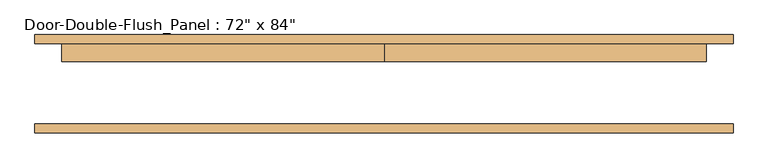
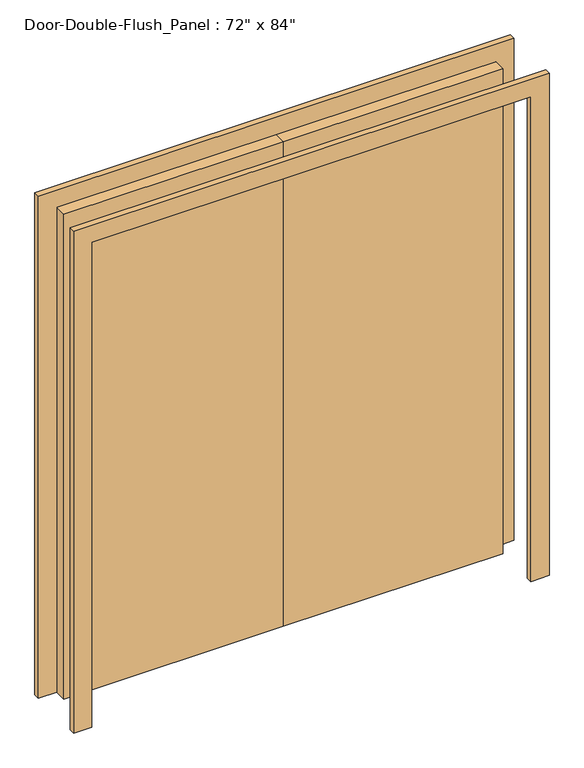
"""IFC4 building model written with IfcOpenShell, lengths in millimetres: door geometry."""

from ifc_helpers import new_model, si_unit, frame, origin, origin_with_axes, place, context, project, spatial, polyline, outline, extrude, source, transform, mapped, element, save


def door_963c5960(model_context):
    return source(origin(), model_context, "Body", "SweptSolid", [
        extrude(outline(polyline([(2133.6, -914.4), (2133.6, 914.4), (0.0, 914.4), (0.0, 990.6), (2209.8, 990.6), (2209.8, -990.6), (0.0, -990.6), (0.0, -914.4), (2133.6, -914.4)])), frame((0.0, 114.3, 0.0), z_axis=(0.0, 1.0, 0.0), x_axis=(0.0, 0.0, 1.0)), (0.0, 0.0, 1.0), 25.4),
        extrude(outline(polyline([(2133.6, -914.4), (2133.6, 914.4), (0.0, 914.4), (0.0, 990.6), (2209.8, 990.6), (2209.8, -990.6), (0.0, -990.6), (0.0, -914.4), (2133.6, -914.4)])), frame((0.0, -139.7, 0.0), z_axis=(0.0, 1.0, 0.0), x_axis=(0.0, 0.0, 1.0)), (0.0, 0.0, 1.0), 25.4),
        extrude(outline(polyline([(-914.4, 114.3), (0.0, 114.3), (0.0, 63.5), (-914.4, 63.5), (-914.4, 114.3)])), origin_with_axes(), (0.0, 0.0, 1.0), 2133.6),
        extrude(outline(polyline([(0.0, 114.3), (914.4, 114.3), (914.4, 63.5), (0.0, 63.5), (0.0, 114.3)])), origin_with_axes(), (0.0, 0.0, 1.0), 2133.6),
    ])


if __name__ == "__main__":
    model = new_model("IFC4")
    model_context = context("Model", 3, world=origin())
    ifc_project = project(units=[si_unit("LENGTHUNIT", "METRE", prefix="MILLI")], contexts=[model_context])
    site = spatial("IfcSite", under=ifc_project)
    building = spatial("IfcBuilding", under=site)
    placement = place(None, origin())
    door_shape = door_963c5960(model_context)
    element("IfcDoor", 1, ObjectType="Door-Double-Flush_Panel : 72\" x 84\"", at=placement, inside=building, context=model_context, shape_type="MappedRepresentation", body=[
        mapped(door_shape, transform((0.0, 0.0, 0.0), x_axis=(1.0, 0.0, 0.0), y_axis=(0.0, 1.0, 0.0), z_axis=(0.0, 0.0, 1.0))),
    ])
    save(model, "model.ifc")

# Revit data of these elements
# Type "Door-Double-Flush_Panel : 72\" x 84\""
#   Type Mark = "16"
#   Construction Type Id = "DOOR"
#   Assembly Code = "C1020"
#   Analytic Construction = "Wooden"
#   Thickness = 0' - 2"
#   Thermal Resistance (R) = 2.5876 (h·ft²·°F)/BTU
#   Swing Angle [instance default] = 90.00°
#   Panel Width = 3' - 0"
#   Heat Transfer Coefficient (U) = 0.3865 BTU/(h·ft²·°F)
#   Height = 7' - 0"
#   Trim Projection Ext = 0' - 1"
#   Trim Projection Int = 0' - 1"
#   Trim Width = 0' - 3"
#   Width = 6' - 0"
#   Define Thermal Properties by = 1
#   Panel Material = Wood - Birch - Solid Stained Light Low Gloss
#   Trim Material = Paint - Sienna
#   Visual Light Transmittance = 0
#   Solar Heat Gain Coefficient = 0
#   Function = (empty or 0)
#   Wall Closure = (empty or 0)
# Element 1 (IfcDoor, "Door-Double-Flush_Panel : 72\" x 84\"")
#   Materials on its faces: "Paint - Sienna", "Wood - Birch - Solid Stained Light Low Gloss"
# Materials
#   "Wood - Birch - Solid Stained Light Low Gloss": class "Wood", colour RGB 210 159 95, transparency 0, Cost = 0
#   "Paint - Sienna": colour RGB 118 70 51, transparency 0, Cost = 0
